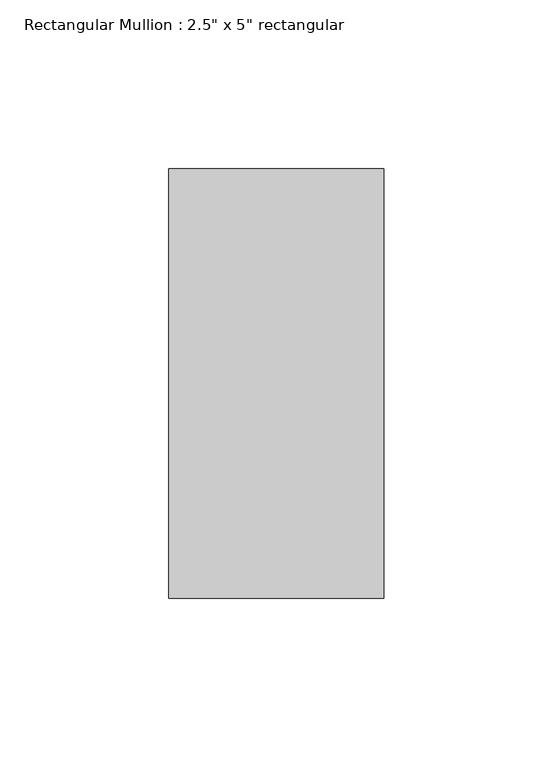
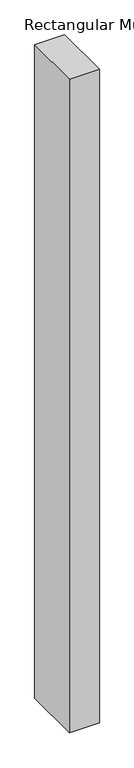
"""IFC4 building model written with IfcOpenShell, lengths in millimetres: member geometry."""

from ifc_helpers import new_model, si_unit, frame, origin, place, context, project, spatial, polyline, outline, extrude, source, transform, mapped, element, save


def member_d09add03(model_context):
    return source(origin(), model_context, "Body", "SweptSolid", [
        extrude(outline(polyline([(0.0, 63.5), (0.0, -63.5), (-63.5, -63.5), (-63.5, 63.5), (0.0, 63.5)])), frame((0.0, 0.0, -1462.4986146), z_axis=(0.0, 0.0, 1.0), x_axis=(1.0, 0.0, 0.0)), (0.0, 0.0, 1.0), 1462.4986146),
    ])


if __name__ == "__main__":
    model = new_model("IFC4")
    model_context = context("Model", 3, world=origin())
    ifc_project = project(units=[si_unit("LENGTHUNIT", "METRE", prefix="MILLI")], contexts=[model_context])
    site = spatial("IfcSite", under=ifc_project)
    building = spatial("IfcBuilding", under=site)
    placement = place(None, origin())
    member_shape = member_d09add03(model_context)
    element("IfcMember", 1, ObjectType="Rectangular Mullion : 2.5\" x 5\" rectangular", at=placement, inside=building, context=model_context, shape_type="MappedRepresentation", body=[
        mapped(member_shape, transform((0.0, 0.0, 0.0), x_axis=(1.0, 0.0, 0.0), y_axis=(0.0, 1.0, 0.0), z_axis=(0.0, 0.0, 1.0))),
    ])
    save(model, "model.ifc")

# Revit data of these elements
# Type "Rectangular Mullion : 2.5\" x 5\" rectangular"
#   built-in parameter 1007304 = 0.416667 (stored number, unit not read)
#   built-in parameter 1007301 = 0.104167 (stored number, unit not read)
#   built-in parameter 1007300 = 0.104167 (stored number, unit not read)
# Element 1 (IfcMember, "Rectangular Mullion : 2.5\" x 5\" rectangular")
#   Materials on its faces: "Aluminum"
# Materials
#   "Aluminum": class "Metal", colour RGB 247 247 247, transparency 0, Description = "Aluminum 6061", Cost = 0
